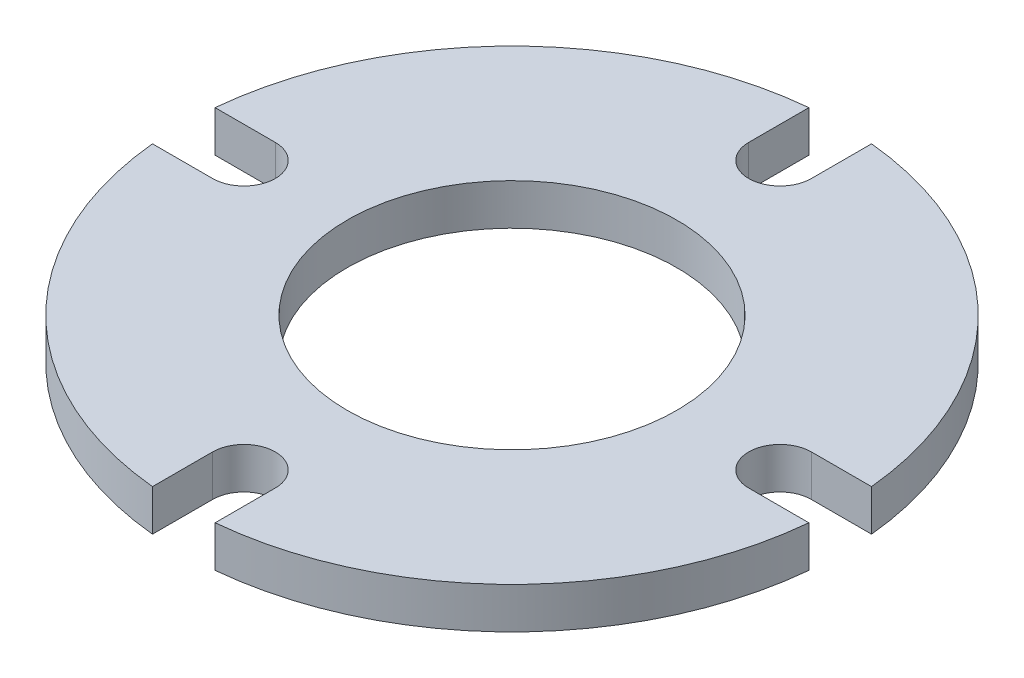
ISO-10303-21;
HEADER;
FILE_DESCRIPTION(('STEP AP214'),'2;1');
FILE_NAME('part.step','',(''),(''),'','','');
FILE_SCHEMA(('AUTOMOTIVE_DESIGN { 1 0 10303 214 1 1 1 1 }'));
ENDSEC;
DATA;
#1=APPLICATION_CONTEXT('core data for automotive mechanical design processes');
#2=APPLICATION_PROTOCOL_DEFINITION('international standard','automotive_design',2000,#1);
#3=PRODUCT_CONTEXT('',#1,'mechanical');
#4=PRODUCT('Part','Part','',(#3));
#5=PRODUCT_RELATED_PRODUCT_CATEGORY('part','',(#4));
#6=PRODUCT_DEFINITION_FORMATION('','',#4);
#7=PRODUCT_DEFINITION_CONTEXT('part definition',#1,'design');
#8=PRODUCT_DEFINITION('design','',#6,#7);
#9=PRODUCT_DEFINITION_SHAPE('','',#8);
#10=(LENGTH_UNIT() NAMED_UNIT(*) SI_UNIT(.MILLI.,.METRE.));
#11=(NAMED_UNIT(*) PLANE_ANGLE_UNIT() SI_UNIT($,.RADIAN.));
#12=(NAMED_UNIT(*) SI_UNIT($,.STERADIAN.) SOLID_ANGLE_UNIT());
#13=UNCERTAINTY_MEASURE_WITH_UNIT(LENGTH_MEASURE(1.E-05),#10,'distance_accuracy_value','');
#14=(GEOMETRIC_REPRESENTATION_CONTEXT(3) GLOBAL_UNCERTAINTY_ASSIGNED_CONTEXT((#13)) GLOBAL_UNIT_ASSIGNED_CONTEXT((#10,
#11,#12)) REPRESENTATION_CONTEXT('',''));
#15=CARTESIAN_POINT('',(0.,0.,0.));
#16=DIRECTION('',(0.,0.,1.));
#17=DIRECTION('',(1.,0.,0.));
#18=AXIS2_PLACEMENT_3D('',#15,#16,#17);
#19=CARTESIAN_POINT('',(0.,6.25,-81.3));
#20=DIRECTION('',(0.,1.,0.));
#21=DIRECTION('',(0.,0.,1.));
#22=AXIS2_PLACEMENT_3D('',#19,#20,#21);
#23=PLANE('',#22);
#24=CARTESIAN_POINT('',(0.,6.25,-81.3));
#25=DIRECTION('',(0.,-1.,0.));
#26=DIRECTION('',(0.,0.,1.));
#27=AXIS2_PLACEMENT_3D('',#24,#25,#26);
#28=CIRCLE('',#27,9.5);
#29=CARTESIAN_POINT('',(9.5,6.25,-81.3));
#30=VERTEX_POINT('',#29);
#31=CARTESIAN_POINT('',(-9.5,6.25,-81.3));
#32=VERTEX_POINT('',#31);
#33=EDGE_CURVE('E214',#30,#32,#28,.T.);
#34=ORIENTED_EDGE('',*,*,#33,.T.);
#35=DIRECTION('',(0.,0.,-1.));
#36=VECTOR('',#35,1.);
#37=CARTESIAN_POINT('',(-9.5,6.25,-81.3));
#38=LINE('',#37,#36);
#39=CARTESIAN_POINT('',(-9.49999999999998,6.25,-99.5477272467835));
#40=VERTEX_POINT('',#39);
#41=EDGE_CURVE('E125',#32,#40,#38,.T.);
#42=ORIENTED_EDGE('',*,*,#41,.T.);
#43=CARTESIAN_POINT('',(0.,6.25,0.));
#44=DIRECTION('',(0.,1.,0.));
#45=DIRECTION('',(0.,0.,1.));
#46=AXIS2_PLACEMENT_3D('',#43,#44,#45);
#47=CIRCLE('',#46,100.);
#48=CARTESIAN_POINT('',(-99.5477272467835,6.25,-9.49999999999996));
#49=VERTEX_POINT('',#48);
#50=EDGE_CURVE('E255',#40,#49,#47,.T.);
#51=ORIENTED_EDGE('',*,*,#50,.T.);
#52=DIRECTION('',(1.,0.,0.));
#53=VECTOR('',#52,1.);
#54=CARTESIAN_POINT('',(-81.3,6.25,-9.49999999999998));
#55=LINE('',#54,#53);
#56=CARTESIAN_POINT('',(-81.3,6.25,-9.49999999999998));
#57=VERTEX_POINT('',#56);
#58=EDGE_CURVE('E272',#49,#57,#55,.T.);
#59=ORIENTED_EDGE('',*,*,#58,.T.);
#60=CARTESIAN_POINT('',(-81.3,6.25,-8.5157229854384E-13));
#61=DIRECTION('',(0.,-1.,0.));
#62=DIRECTION('',(0.,0.,1.));
#63=AXIS2_PLACEMENT_3D('',#60,#61,#62);
#64=CIRCLE('',#63,9.5);
#65=CARTESIAN_POINT('',(-81.3,6.25,9.49999999999914));
#66=VERTEX_POINT('',#65);
#67=EDGE_CURVE('E269',#57,#66,#64,.T.);
#68=ORIENTED_EDGE('',*,*,#67,.T.);
#69=DIRECTION('',(-1.,0.,0.));
#70=VECTOR('',#69,1.);
#71=CARTESIAN_POINT('',(-81.3,6.25,9.50000000000001));
#72=LINE('',#71,#70);
#73=CARTESIAN_POINT('',(-99.5477272467835,6.25,9.5));
#74=VERTEX_POINT('',#73);
#75=EDGE_CURVE('E275',#66,#74,#72,.T.);
#76=ORIENTED_EDGE('',*,*,#75,.T.);
#77=CARTESIAN_POINT('',(0.,6.25,0.));
#78=DIRECTION('',(0.,1.,0.));
#79=DIRECTION('',(0.,0.,1.));
#80=AXIS2_PLACEMENT_3D('',#77,#78,#79);
#81=CIRCLE('',#80,100.);
#82=CARTESIAN_POINT('',(-9.49999999999996,6.25,99.5477272467835));
#83=VERTEX_POINT('',#82);
#84=EDGE_CURVE('E274',#74,#83,#81,.T.);
#85=ORIENTED_EDGE('',*,*,#84,.T.);
#86=DIRECTION('',(0.,0.,-1.));
#87=VECTOR('',#86,1.);
#88=CARTESIAN_POINT('',(-9.49999999999999,6.25,81.3));
#89=LINE('',#88,#87);
#90=CARTESIAN_POINT('',(-9.49999999999999,6.25,81.3));
#91=VERTEX_POINT('',#90);
#92=EDGE_CURVE('E282',#83,#91,#89,.T.);
#93=ORIENTED_EDGE('',*,*,#92,.T.);
#94=CARTESIAN_POINT('',(-5.67714865695893E-13,6.25,81.3));
#95=DIRECTION('',(0.,-1.,0.));
#96=DIRECTION('',(0.,0.,1.));
#97=AXIS2_PLACEMENT_3D('',#94,#95,#96);
#98=CIRCLE('',#97,9.49999999999999);
#99=CARTESIAN_POINT('',(9.49999999999943,6.25,81.3));
#100=VERTEX_POINT('',#99);
#101=EDGE_CURVE('E284',#91,#100,#98,.T.);
#102=ORIENTED_EDGE('',*,*,#101,.T.);
#103=DIRECTION('',(0.,0.,1.));
#104=VECTOR('',#103,1.);
#105=CARTESIAN_POINT('',(9.50000000000001,6.25,81.3));
#106=LINE('',#105,#104);
#107=CARTESIAN_POINT('',(9.49999999999999,6.25,99.5477272467835));
#108=VERTEX_POINT('',#107);
#109=EDGE_CURVE('E283',#100,#108,#106,.T.);
#110=ORIENTED_EDGE('',*,*,#109,.T.);
#111=CARTESIAN_POINT('',(0.,6.25,0.));
#112=DIRECTION('',(0.,1.,0.));
#113=DIRECTION('',(0.,0.,1.));
#114=AXIS2_PLACEMENT_3D('',#111,#112,#113);
#115=CIRCLE('',#114,100.);
#116=CARTESIAN_POINT('',(99.5477272467835,6.25,9.49999999999997));
#117=VERTEX_POINT('',#116);
#118=EDGE_CURVE('E289',#108,#117,#115,.T.);
#119=ORIENTED_EDGE('',*,*,#118,.T.);
#120=DIRECTION('',(-1.,0.,0.));
#121=VECTOR('',#120,1.);
#122=CARTESIAN_POINT('',(81.3,6.25,9.49999999999999));
#123=LINE('',#122,#121);
#124=CARTESIAN_POINT('',(81.3,6.25,9.49999999999999));
#125=VERTEX_POINT('',#124);
#126=EDGE_CURVE('E286',#117,#125,#123,.T.);
#127=ORIENTED_EDGE('',*,*,#126,.T.);
#128=CARTESIAN_POINT('',(81.3,6.25,2.83857432847947E-13));
#129=DIRECTION('',(0.,-1.,0.));
#130=DIRECTION('',(0.,0.,1.));
#131=AXIS2_PLACEMENT_3D('',#128,#129,#130);
#132=CIRCLE('',#131,9.5);
#133=CARTESIAN_POINT('',(81.3,6.25,-9.49999999999971));
#134=VERTEX_POINT('',#133);
#135=EDGE_CURVE('E167',#125,#134,#132,.T.);
#136=ORIENTED_EDGE('',*,*,#135,.T.);
#137=DIRECTION('',(1.,0.,0.));
#138=VECTOR('',#137,1.);
#139=CARTESIAN_POINT('',(81.3,6.25,-9.5));
#140=LINE('',#139,#138);
#141=CARTESIAN_POINT('',(99.5477272467835,6.25,-9.49999999999999));
#142=VERTEX_POINT('',#141);
#143=EDGE_CURVE('E159',#134,#142,#140,.T.);
#144=ORIENTED_EDGE('',*,*,#143,.T.);
#145=CARTESIAN_POINT('',(0.,6.25,0.));
#146=DIRECTION('',(0.,1.,0.));
#147=DIRECTION('',(0.,0.,1.));
#148=AXIS2_PLACEMENT_3D('',#145,#146,#147);
#149=CIRCLE('',#148,100.);
#150=CARTESIAN_POINT('',(9.49999999999999,6.25,-99.5477272467835));
#151=VERTEX_POINT('',#150);
#152=EDGE_CURVE('E163',#142,#151,#149,.T.);
#153=ORIENTED_EDGE('',*,*,#152,.T.);
#154=DIRECTION('',(0.,0.,1.));
#155=VECTOR('',#154,1.);
#156=CARTESIAN_POINT('',(9.5,6.25,-81.3));
#157=LINE('',#156,#155);
#158=EDGE_CURVE('E57',#151,#30,#157,.T.);
#159=ORIENTED_EDGE('',*,*,#158,.T.);
#160=EDGE_LOOP('',(#34,#42,#51,#59,#68,#76,#85,#93,#102,#110,#119,#127,#136,#144,#153,#159));
#161=FACE_BOUND('',#160,.T.);
#162=CARTESIAN_POINT('',(0.,6.25,0.));
#163=DIRECTION('',(0.,1.,0.));
#164=DIRECTION('',(0.,0.,1.));
#165=AXIS2_PLACEMENT_3D('',#162,#163,#164);
#166=CIRCLE('',#165,50.);
#167=CARTESIAN_POINT('',(0.,6.25,50.));
#168=VERTEX_POINT('',#167);
#169=EDGE_CURVE('E189',#168,#168,#166,.T.);
#170=ORIENTED_EDGE('',*,*,#169,.F.);
#171=EDGE_LOOP('',(#170));
#172=FACE_BOUND('',#171,.T.);
#173=ADVANCED_FACE('F39',(#161,#172),#23,.T.);
#174=CARTESIAN_POINT('',(0.,-6.25,-81.3));
#175=DIRECTION('',(0.,1.,0.));
#176=DIRECTION('',(0.,0.,1.));
#177=AXIS2_PLACEMENT_3D('',#174,#175,#176);
#178=PLANE('',#177);
#179=CARTESIAN_POINT('',(0.,-6.25,-81.3));
#180=DIRECTION('',(0.,-1.,0.));
#181=DIRECTION('',(0.,0.,1.));
#182=AXIS2_PLACEMENT_3D('',#179,#180,#181);
#183=CIRCLE('',#182,9.5);
#184=CARTESIAN_POINT('',(9.5,-6.25,-81.3));
#185=VERTEX_POINT('',#184);
#186=CARTESIAN_POINT('',(-9.5,-6.25,-81.3));
#187=VERTEX_POINT('',#186);
#188=EDGE_CURVE('E184',#185,#187,#183,.T.);
#189=ORIENTED_EDGE('',*,*,#188,.F.);
#190=DIRECTION('',(0.,0.,1.));
#191=VECTOR('',#190,1.);
#192=CARTESIAN_POINT('',(9.5,-6.25,-81.3));
#193=LINE('',#192,#191);
#194=CARTESIAN_POINT('',(9.49999999999999,-6.25,-99.5477272467835));
#195=VERTEX_POINT('',#194);
#196=EDGE_CURVE('E113',#195,#185,#193,.T.);
#197=ORIENTED_EDGE('',*,*,#196,.F.);
#198=CARTESIAN_POINT('',(0.,-6.25,0.));
#199=DIRECTION('',(0.,1.,0.));
#200=DIRECTION('',(0.,0.,1.));
#201=AXIS2_PLACEMENT_3D('',#198,#199,#200);
#202=CIRCLE('',#201,100.);
#203=CARTESIAN_POINT('',(99.5477272467835,-6.25,-9.49999999999999));
#204=VERTEX_POINT('',#203);
#205=EDGE_CURVE('E108',#204,#195,#202,.T.);
#206=ORIENTED_EDGE('',*,*,#205,.F.);
#207=DIRECTION('',(1.,0.,0.));
#208=VECTOR('',#207,1.);
#209=CARTESIAN_POINT('',(81.3,-6.25,-9.5));
#210=LINE('',#209,#208);
#211=CARTESIAN_POINT('',(81.3,-6.25,-9.49999999999971));
#212=VERTEX_POINT('',#211);
#213=EDGE_CURVE('E171',#212,#204,#210,.T.);
#214=ORIENTED_EDGE('',*,*,#213,.F.);
#215=CARTESIAN_POINT('',(81.3,-6.25,2.83857432847947E-13));
#216=DIRECTION('',(0.,-1.,0.));
#217=DIRECTION('',(0.,0.,1.));
#218=AXIS2_PLACEMENT_3D('',#215,#216,#217);
#219=CIRCLE('',#218,9.5);
#220=CARTESIAN_POINT('',(81.3,-6.25,9.49999999999999));
#221=VERTEX_POINT('',#220);
#222=EDGE_CURVE('E209',#221,#212,#219,.T.);
#223=ORIENTED_EDGE('',*,*,#222,.F.);
#224=DIRECTION('',(-1.,0.,0.));
#225=VECTOR('',#224,1.);
#226=CARTESIAN_POINT('',(81.3,-6.25,9.49999999999999));
#227=LINE('',#226,#225);
#228=CARTESIAN_POINT('',(99.5477272467835,-6.25,9.49999999999997));
#229=VERTEX_POINT('',#228);
#230=EDGE_CURVE('E208',#229,#221,#227,.T.);
#231=ORIENTED_EDGE('',*,*,#230,.F.);
#232=CARTESIAN_POINT('',(0.,-6.25,0.));
#233=DIRECTION('',(0.,1.,0.));
#234=DIRECTION('',(0.,0.,1.));
#235=AXIS2_PLACEMENT_3D('',#232,#233,#234);
#236=CIRCLE('',#235,100.);
#237=CARTESIAN_POINT('',(9.49999999999999,-6.25,99.5477272467835));
#238=VERTEX_POINT('',#237);
#239=EDGE_CURVE('E206',#238,#229,#236,.T.);
#240=ORIENTED_EDGE('',*,*,#239,.F.);
#241=DIRECTION('',(0.,0.,1.));
#242=VECTOR('',#241,1.);
#243=CARTESIAN_POINT('',(9.50000000000001,-6.25,81.3));
#244=LINE('',#243,#242);
#245=CARTESIAN_POINT('',(9.49999999999943,-6.25,81.3));
#246=VERTEX_POINT('',#245);
#247=EDGE_CURVE('E204',#246,#238,#244,.T.);
#248=ORIENTED_EDGE('',*,*,#247,.F.);
#249=CARTESIAN_POINT('',(-5.67714865695893E-13,-6.25,81.3));
#250=DIRECTION('',(0.,-1.,0.));
#251=DIRECTION('',(0.,0.,1.));
#252=AXIS2_PLACEMENT_3D('',#249,#250,#251);
#253=CIRCLE('',#252,9.49999999999999);
#254=CARTESIAN_POINT('',(-9.49999999999999,-6.25,81.3));
#255=VERTEX_POINT('',#254);
#256=EDGE_CURVE('E205',#255,#246,#253,.T.);
#257=ORIENTED_EDGE('',*,*,#256,.F.);
#258=DIRECTION('',(0.,0.,-1.));
#259=VECTOR('',#258,1.);
#260=CARTESIAN_POINT('',(-9.49999999999999,-6.25,81.3));
#261=LINE('',#260,#259);
#262=CARTESIAN_POINT('',(-9.49999999999996,-6.25,99.5477272467835));
#263=VERTEX_POINT('',#262);
#264=EDGE_CURVE('E199',#263,#255,#261,.T.);
#265=ORIENTED_EDGE('',*,*,#264,.F.);
#266=CARTESIAN_POINT('',(0.,-6.25,0.));
#267=DIRECTION('',(0.,1.,0.));
#268=DIRECTION('',(0.,0.,1.));
#269=AXIS2_PLACEMENT_3D('',#266,#267,#268);
#270=CIRCLE('',#269,100.);
#271=CARTESIAN_POINT('',(-99.5477272467835,-6.25,9.5));
#272=VERTEX_POINT('',#271);
#273=EDGE_CURVE('E196',#272,#263,#270,.T.);
#274=ORIENTED_EDGE('',*,*,#273,.F.);
#275=DIRECTION('',(-1.,0.,0.));
#276=VECTOR('',#275,1.);
#277=CARTESIAN_POINT('',(-81.3,-6.25,9.50000000000001));
#278=LINE('',#277,#276);
#279=CARTESIAN_POINT('',(-81.3,-6.25,9.49999999999914));
#280=VERTEX_POINT('',#279);
#281=EDGE_CURVE('E198',#280,#272,#278,.T.);
#282=ORIENTED_EDGE('',*,*,#281,.F.);
#283=CARTESIAN_POINT('',(-81.3,-6.25,-8.5157229854384E-13));
#284=DIRECTION('',(0.,-1.,0.));
#285=DIRECTION('',(0.,0.,1.));
#286=AXIS2_PLACEMENT_3D('',#283,#284,#285);
#287=CIRCLE('',#286,9.5);
#288=CARTESIAN_POINT('',(-81.3,-6.25,-9.49999999999998));
#289=VERTEX_POINT('',#288);
#290=EDGE_CURVE('E191',#289,#280,#287,.T.);
#291=ORIENTED_EDGE('',*,*,#290,.F.);
#292=DIRECTION('',(1.,0.,0.));
#293=VECTOR('',#292,1.);
#294=CARTESIAN_POINT('',(-81.3,-6.25,-9.49999999999998));
#295=LINE('',#294,#293);
#296=CARTESIAN_POINT('',(-99.5477272467835,-6.25,-9.49999999999996));
#297=VERTEX_POINT('',#296);
#298=EDGE_CURVE('E194',#297,#289,#295,.T.);
#299=ORIENTED_EDGE('',*,*,#298,.F.);
#300=CARTESIAN_POINT('',(0.,-6.25,0.));
#301=DIRECTION('',(0.,1.,0.));
#302=DIRECTION('',(0.,0.,1.));
#303=AXIS2_PLACEMENT_3D('',#300,#301,#302);
#304=CIRCLE('',#303,100.);
#305=CARTESIAN_POINT('',(-9.49999999999998,-6.25,-99.5477272467835));
#306=VERTEX_POINT('',#305);
#307=EDGE_CURVE('E188',#306,#297,#304,.T.);
#308=ORIENTED_EDGE('',*,*,#307,.F.);
#309=DIRECTION('',(0.,0.,-1.));
#310=VECTOR('',#309,1.);
#311=CARTESIAN_POINT('',(-9.5,-6.25,-81.3));
#312=LINE('',#311,#310);
#313=EDGE_CURVE('E190',#187,#306,#312,.T.);
#314=ORIENTED_EDGE('',*,*,#313,.F.);
#315=EDGE_LOOP('',(#189,#197,#206,#214,#223,#231,#240,#248,#257,#265,#274,#282,#291,#299,#308,#314));
#316=FACE_BOUND('',#315,.T.);
#317=CARTESIAN_POINT('',(0.,-6.25,0.));
#318=DIRECTION('',(0.,1.,0.));
#319=DIRECTION('',(0.,0.,1.));
#320=AXIS2_PLACEMENT_3D('',#317,#318,#319);
#321=CIRCLE('',#320,50.);
#322=CARTESIAN_POINT('',(0.,-6.25,50.));
#323=VERTEX_POINT('',#322);
#324=EDGE_CURVE('E488',#323,#323,#321,.T.);
#325=ORIENTED_EDGE('',*,*,#324,.T.);
#326=EDGE_LOOP('',(#325));
#327=FACE_BOUND('',#326,.T.);
#328=ADVANCED_FACE('F256',(#316,#327),#178,.F.);
#329=CARTESIAN_POINT('',(0.,6.25,-81.3));
#330=DIRECTION('',(0.,-1.,0.));
#331=DIRECTION('',(0.,0.,-1.));
#332=AXIS2_PLACEMENT_3D('',#329,#330,#331);
#333=CYLINDRICAL_SURFACE('',#332,9.5);
#334=ORIENTED_EDGE('',*,*,#188,.T.);
#335=DIRECTION('',(0.,-1.,0.));
#336=VECTOR('',#335,1.);
#337=CARTESIAN_POINT('',(-9.5,6.25,-81.3));
#338=LINE('',#337,#336);
#339=EDGE_CURVE('E11',#32,#187,#338,.T.);
#340=ORIENTED_EDGE('',*,*,#339,.F.);
#341=ORIENTED_EDGE('',*,*,#33,.F.);
#342=DIRECTION('',(0.,-1.,0.));
#343=VECTOR('',#342,1.);
#344=CARTESIAN_POINT('',(9.5,6.25,-81.3));
#345=LINE('',#344,#343);
#346=EDGE_CURVE('E178',#30,#185,#345,.T.);
#347=ORIENTED_EDGE('',*,*,#346,.T.);
#348=EDGE_LOOP('',(#334,#340,#341,#347));
#349=FACE_BOUND('',#348,.T.);
#350=ADVANCED_FACE('F41',(#349),#333,.F.);
#351=CARTESIAN_POINT('',(-9.5,6.25,-81.3));
#352=DIRECTION('',(-1.,0.,0.));
#353=DIRECTION('',(0.,0.,1.));
#354=AXIS2_PLACEMENT_3D('',#351,#352,#353);
#355=PLANE('',#354);
#356=ORIENTED_EDGE('',*,*,#313,.T.);
#357=DIRECTION('',(0.,-1.,0.));
#358=VECTOR('',#357,1.);
#359=CARTESIAN_POINT('',(-9.49999999999998,6.25,-99.5477272467835));
#360=LINE('',#359,#358);
#361=EDGE_CURVE('E48',#40,#306,#360,.T.);
#362=ORIENTED_EDGE('',*,*,#361,.F.);
#363=ORIENTED_EDGE('',*,*,#41,.F.);
#364=ORIENTED_EDGE('',*,*,#339,.T.);
#365=EDGE_LOOP('',(#356,#362,#363,#364));
#366=FACE_BOUND('',#365,.T.);
#367=ADVANCED_FACE('F323',(#366),#355,.F.);
#368=CARTESIAN_POINT('',(0.,6.25,0.));
#369=DIRECTION('',(0.,-1.,0.));
#370=DIRECTION('',(0.,0.,-1.));
#371=AXIS2_PLACEMENT_3D('',#368,#369,#370);
#372=CYLINDRICAL_SURFACE('',#371,100.);
#373=ORIENTED_EDGE('',*,*,#307,.T.);
#374=DIRECTION('',(0.,-1.,0.));
#375=VECTOR('',#374,1.);
#376=CARTESIAN_POINT('',(-99.5477272467835,6.25,-9.49999999999996));
#377=LINE('',#376,#375);
#378=EDGE_CURVE('E247',#49,#297,#377,.T.);
#379=ORIENTED_EDGE('',*,*,#378,.F.);
#380=ORIENTED_EDGE('',*,*,#50,.F.);
#381=ORIENTED_EDGE('',*,*,#361,.T.);
#382=EDGE_LOOP('',(#373,#379,#380,#381));
#383=FACE_BOUND('',#382,.T.);
#384=ADVANCED_FACE('F252',(#383),#372,.T.);
#385=CARTESIAN_POINT('',(-81.3,6.25,-9.49999999999998));
#386=DIRECTION('',(0.,0.,-1.));
#387=DIRECTION('',(-1.,0.,0.));
#388=AXIS2_PLACEMENT_3D('',#385,#386,#387);
#389=PLANE('',#388);
#390=ORIENTED_EDGE('',*,*,#298,.T.);
#391=DIRECTION('',(0.,-1.,0.));
#392=VECTOR('',#391,1.);
#393=CARTESIAN_POINT('',(-81.3,6.25,-9.49999999999998));
#394=LINE('',#393,#392);
#395=EDGE_CURVE('E244',#57,#289,#394,.T.);
#396=ORIENTED_EDGE('',*,*,#395,.F.);
#397=ORIENTED_EDGE('',*,*,#58,.F.);
#398=ORIENTED_EDGE('',*,*,#378,.T.);
#399=EDGE_LOOP('',(#390,#396,#397,#398));
#400=FACE_BOUND('',#399,.T.);
#401=ADVANCED_FACE('F262',(#400),#389,.F.);
#402=CARTESIAN_POINT('',(-81.3,6.25,-8.5157229854384E-13));
#403=DIRECTION('',(0.,-1.,0.));
#404=DIRECTION('',(0.,0.,-1.));
#405=AXIS2_PLACEMENT_3D('',#402,#403,#404);
#406=CYLINDRICAL_SURFACE('',#405,9.5);
#407=ORIENTED_EDGE('',*,*,#290,.T.);
#408=DIRECTION('',(0.,-1.,0.));
#409=VECTOR('',#408,1.);
#410=CARTESIAN_POINT('',(-81.3,6.25,9.49999999999914));
#411=LINE('',#410,#409);
#412=EDGE_CURVE('E238',#66,#280,#411,.T.);
#413=ORIENTED_EDGE('',*,*,#412,.F.);
#414=ORIENTED_EDGE('',*,*,#67,.F.);
#415=ORIENTED_EDGE('',*,*,#395,.T.);
#416=EDGE_LOOP('',(#407,#413,#414,#415));
#417=FACE_BOUND('',#416,.T.);
#418=ADVANCED_FACE('F268',(#417),#406,.F.);
#419=CARTESIAN_POINT('',(-81.3,6.25,9.50000000000001));
#420=DIRECTION('',(0.,0.,1.));
#421=DIRECTION('',(1.,0.,0.));
#422=AXIS2_PLACEMENT_3D('',#419,#420,#421);
#423=PLANE('',#422);
#424=ORIENTED_EDGE('',*,*,#281,.T.);
#425=DIRECTION('',(0.,-1.,0.));
#426=VECTOR('',#425,1.);
#427=CARTESIAN_POINT('',(-99.5477272467835,6.25,9.5));
#428=LINE('',#427,#426);
#429=EDGE_CURVE('E240',#74,#272,#428,.T.);
#430=ORIENTED_EDGE('',*,*,#429,.F.);
#431=ORIENTED_EDGE('',*,*,#75,.F.);
#432=ORIENTED_EDGE('',*,*,#412,.T.);
#433=EDGE_LOOP('',(#424,#430,#431,#432));
#434=FACE_BOUND('',#433,.T.);
#435=ADVANCED_FACE('F337',(#434),#423,.F.);
#436=CARTESIAN_POINT('',(0.,6.25,0.));
#437=DIRECTION('',(0.,-1.,0.));
#438=DIRECTION('',(0.,0.,-1.));
#439=AXIS2_PLACEMENT_3D('',#436,#437,#438);
#440=CYLINDRICAL_SURFACE('',#439,100.);
#441=ORIENTED_EDGE('',*,*,#273,.T.);
#442=DIRECTION('',(0.,-1.,0.));
#443=VECTOR('',#442,1.);
#444=CARTESIAN_POINT('',(-9.49999999999996,6.25,99.5477272467835));
#445=LINE('',#444,#443);
#446=EDGE_CURVE('E231',#83,#263,#445,.T.);
#447=ORIENTED_EDGE('',*,*,#446,.F.);
#448=ORIENTED_EDGE('',*,*,#84,.F.);
#449=ORIENTED_EDGE('',*,*,#429,.T.);
#450=EDGE_LOOP('',(#441,#447,#448,#449));
#451=FACE_BOUND('',#450,.T.);
#452=ADVANCED_FACE('F336',(#451),#440,.T.);
#453=CARTESIAN_POINT('',(-9.49999999999999,6.25,81.3));
#454=DIRECTION('',(-1.,0.,0.));
#455=DIRECTION('',(0.,0.,1.));
#456=AXIS2_PLACEMENT_3D('',#453,#454,#455);
#457=PLANE('',#456);
#458=ORIENTED_EDGE('',*,*,#264,.T.);
#459=DIRECTION('',(0.,-1.,0.));
#460=VECTOR('',#459,1.);
#461=CARTESIAN_POINT('',(-9.49999999999999,6.25,81.3));
#462=LINE('',#461,#460);
#463=EDGE_CURVE('E232',#91,#255,#462,.T.);
#464=ORIENTED_EDGE('',*,*,#463,.F.);
#465=ORIENTED_EDGE('',*,*,#92,.F.);
#466=ORIENTED_EDGE('',*,*,#446,.T.);
#467=EDGE_LOOP('',(#458,#464,#465,#466));
#468=FACE_BOUND('',#467,.T.);
#469=ADVANCED_FACE('F345',(#468),#457,.F.);
#470=CARTESIAN_POINT('',(-5.67714865695893E-13,6.25,81.3));
#471=DIRECTION('',(0.,-1.,0.));
#472=DIRECTION('',(0.,0.,-1.));
#473=AXIS2_PLACEMENT_3D('',#470,#471,#472);
#474=CYLINDRICAL_SURFACE('',#473,9.49999999999999);
#475=ORIENTED_EDGE('',*,*,#256,.T.);
#476=DIRECTION('',(0.,-1.,0.));
#477=VECTOR('',#476,1.);
#478=CARTESIAN_POINT('',(9.49999999999943,6.25,81.3));
#479=LINE('',#478,#477);
#480=EDGE_CURVE('E229',#100,#246,#479,.T.);
#481=ORIENTED_EDGE('',*,*,#480,.F.);
#482=ORIENTED_EDGE('',*,*,#101,.F.);
#483=ORIENTED_EDGE('',*,*,#463,.T.);
#484=EDGE_LOOP('',(#475,#481,#482,#483));
#485=FACE_BOUND('',#484,.T.);
#486=ADVANCED_FACE('F350',(#485),#474,.F.);
#487=CARTESIAN_POINT('',(9.50000000000001,6.25,81.3));
#488=DIRECTION('',(1.,0.,0.));
#489=DIRECTION('',(0.,0.,-1.));
#490=AXIS2_PLACEMENT_3D('',#487,#488,#489);
#491=PLANE('',#490);
#492=ORIENTED_EDGE('',*,*,#247,.T.);
#493=DIRECTION('',(0.,-1.,0.));
#494=VECTOR('',#493,1.);
#495=CARTESIAN_POINT('',(9.49999999999999,6.25,99.5477272467835));
#496=LINE('',#495,#494);
#497=EDGE_CURVE('E223',#108,#238,#496,.T.);
#498=ORIENTED_EDGE('',*,*,#497,.F.);
#499=ORIENTED_EDGE('',*,*,#109,.F.);
#500=ORIENTED_EDGE('',*,*,#480,.T.);
#501=EDGE_LOOP('',(#492,#498,#499,#500));
#502=FACE_BOUND('',#501,.T.);
#503=ADVANCED_FACE('F352',(#502),#491,.F.);
#504=CARTESIAN_POINT('',(0.,6.25,0.));
#505=DIRECTION('',(0.,-1.,0.));
#506=DIRECTION('',(0.,0.,-1.));
#507=AXIS2_PLACEMENT_3D('',#504,#505,#506);
#508=CYLINDRICAL_SURFACE('',#507,100.);
#509=ORIENTED_EDGE('',*,*,#239,.T.);
#510=DIRECTION('',(0.,-1.,0.));
#511=VECTOR('',#510,1.);
#512=CARTESIAN_POINT('',(99.5477272467835,6.25,9.49999999999997));
#513=LINE('',#512,#511);
#514=EDGE_CURVE('E225',#117,#229,#513,.T.);
#515=ORIENTED_EDGE('',*,*,#514,.F.);
#516=ORIENTED_EDGE('',*,*,#118,.F.);
#517=ORIENTED_EDGE('',*,*,#497,.T.);
#518=EDGE_LOOP('',(#509,#515,#516,#517));
#519=FACE_BOUND('',#518,.T.);
#520=ADVANCED_FACE('F353',(#519),#508,.T.);
#521=CARTESIAN_POINT('',(81.3,6.25,9.49999999999999));
#522=DIRECTION('',(0.,0.,1.));
#523=DIRECTION('',(1.,0.,0.));
#524=AXIS2_PLACEMENT_3D('',#521,#522,#523);
#525=PLANE('',#524);
#526=ORIENTED_EDGE('',*,*,#230,.T.);
#527=DIRECTION('',(0.,-1.,0.));
#528=VECTOR('',#527,1.);
#529=CARTESIAN_POINT('',(81.3,6.25,9.49999999999999));
#530=LINE('',#529,#528);
#531=EDGE_CURVE('E218',#125,#221,#530,.T.);
#532=ORIENTED_EDGE('',*,*,#531,.F.);
#533=ORIENTED_EDGE('',*,*,#126,.F.);
#534=ORIENTED_EDGE('',*,*,#514,.T.);
#535=EDGE_LOOP('',(#526,#532,#533,#534));
#536=FACE_BOUND('',#535,.T.);
#537=ADVANCED_FACE('F293',(#536),#525,.F.);
#538=CARTESIAN_POINT('',(81.3,6.25,2.83857432847947E-13));
#539=DIRECTION('',(0.,-1.,0.));
#540=DIRECTION('',(0.,0.,-1.));
#541=AXIS2_PLACEMENT_3D('',#538,#539,#540);
#542=CYLINDRICAL_SURFACE('',#541,9.5);
#543=ORIENTED_EDGE('',*,*,#222,.T.);
#544=DIRECTION('',(0.,-1.,0.));
#545=VECTOR('',#544,1.);
#546=CARTESIAN_POINT('',(81.3,6.25,-9.49999999999971));
#547=LINE('',#546,#545);
#548=EDGE_CURVE('E173',#134,#212,#547,.T.);
#549=ORIENTED_EDGE('',*,*,#548,.F.);
#550=ORIENTED_EDGE('',*,*,#135,.F.);
#551=ORIENTED_EDGE('',*,*,#531,.T.);
#552=EDGE_LOOP('',(#543,#549,#550,#551));
#553=FACE_BOUND('',#552,.T.);
#554=ADVANCED_FACE('F296',(#553),#542,.F.);
#555=CARTESIAN_POINT('',(81.3,6.25,-9.5));
#556=DIRECTION('',(0.,0.,-1.));
#557=DIRECTION('',(-1.,0.,0.));
#558=AXIS2_PLACEMENT_3D('',#555,#556,#557);
#559=PLANE('',#558);
#560=ORIENTED_EDGE('',*,*,#213,.T.);
#561=DIRECTION('',(0.,-1.,0.));
#562=VECTOR('',#561,1.);
#563=CARTESIAN_POINT('',(99.5477272467835,6.25,-9.49999999999999));
#564=LINE('',#563,#562);
#565=EDGE_CURVE('E172',#142,#204,#564,.T.);
#566=ORIENTED_EDGE('',*,*,#565,.F.);
#567=ORIENTED_EDGE('',*,*,#143,.F.);
#568=ORIENTED_EDGE('',*,*,#548,.T.);
#569=EDGE_LOOP('',(#560,#566,#567,#568));
#570=FACE_BOUND('',#569,.T.);
#571=ADVANCED_FACE('F175',(#570),#559,.F.);
#572=CARTESIAN_POINT('',(0.,6.25,0.));
#573=DIRECTION('',(0.,-1.,0.));
#574=DIRECTION('',(0.,0.,-1.));
#575=AXIS2_PLACEMENT_3D('',#572,#573,#574);
#576=CYLINDRICAL_SURFACE('',#575,100.);
#577=ORIENTED_EDGE('',*,*,#205,.T.);
#578=DIRECTION('',(0.,-1.,0.));
#579=VECTOR('',#578,1.);
#580=CARTESIAN_POINT('',(9.49999999999999,6.25,-99.5477272467835));
#581=LINE('',#580,#579);
#582=EDGE_CURVE('E177',#151,#195,#581,.T.);
#583=ORIENTED_EDGE('',*,*,#582,.F.);
#584=ORIENTED_EDGE('',*,*,#152,.F.);
#585=ORIENTED_EDGE('',*,*,#565,.T.);
#586=EDGE_LOOP('',(#577,#583,#584,#585));
#587=FACE_BOUND('',#586,.T.);
#588=ADVANCED_FACE('F180',(#587),#576,.T.);
#589=CARTESIAN_POINT('',(9.5,6.25,-81.3));
#590=DIRECTION('',(1.,0.,0.));
#591=DIRECTION('',(0.,0.,-1.));
#592=AXIS2_PLACEMENT_3D('',#589,#590,#591);
#593=PLANE('',#592);
#594=ORIENTED_EDGE('',*,*,#196,.T.);
#595=ORIENTED_EDGE('',*,*,#346,.F.);
#596=ORIENTED_EDGE('',*,*,#158,.F.);
#597=ORIENTED_EDGE('',*,*,#582,.T.);
#598=EDGE_LOOP('',(#594,#595,#596,#597));
#599=FACE_BOUND('',#598,.T.);
#600=ADVANCED_FACE('F305',(#599),#593,.F.);
#601=CARTESIAN_POINT('',(0.,6.25,0.));
#602=DIRECTION('',(0.,-1.,0.));
#603=DIRECTION('',(0.,0.,-1.));
#604=AXIS2_PLACEMENT_3D('',#601,#602,#603);
#605=CYLINDRICAL_SURFACE('',#604,50.);
#606=ORIENTED_EDGE('',*,*,#169,.T.);
#607=EDGE_LOOP('',(#606));
#608=FACE_BOUND('',#607,.T.);
#609=ORIENTED_EDGE('',*,*,#324,.F.);
#610=EDGE_LOOP('',(#609));
#611=FACE_BOUND('',#610,.T.);
#612=ADVANCED_FACE('F303',(#608,#611),#605,.F.);
#613=CLOSED_SHELL('',(#173,#328,#350,#367,#384,#401,#418,#435,#452,#469,#486,#503,#520,#537,
#554,#571,#588,#600,#612));
#614=MANIFOLD_SOLID_BREP('B2',#613);
#615=ADVANCED_BREP_SHAPE_REPRESENTATION('',(#18,#614),#14);
#616=SHAPE_DEFINITION_REPRESENTATION(#9,#615);
ENDSEC;
END-ISO-10303-21;
